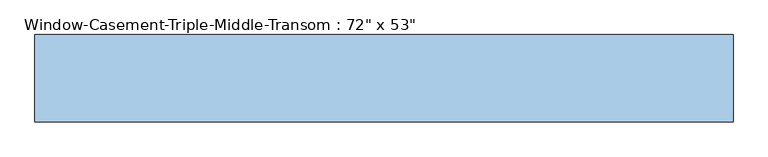
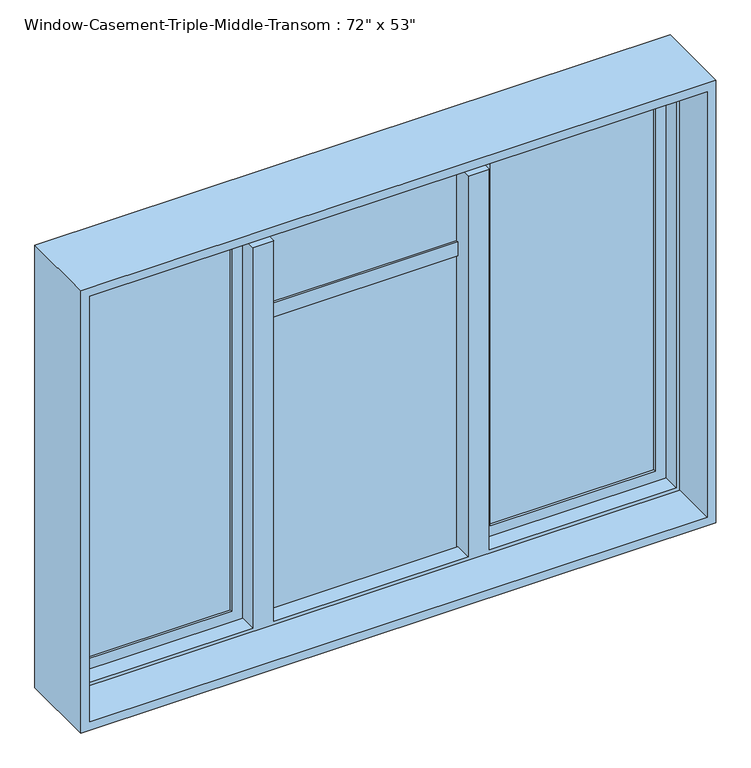
"""IFC4 building model written with IfcOpenShell, lengths in millimetres: window geometry."""

from ifc_helpers import new_model, si_unit, frame, origin, place, context, project, spatial, polyline, outline, extrude, faceted_brep, source, transform, mapped, element, save


def window_7a1f68bc(model_context):
    return source(origin(), model_context, "Body", "SolidModel", [
        extrude(outline(polyline([(2235.2, 330.2), (939.8, 330.2), (939.8, 889.0), (2235.2, 889.0), (2235.2, 330.2)]), holes=[polyline([(2193.3296875, 847.1296875), (981.6703125, 847.1296875), (981.6703125, 372.0703125), (2193.3296875, 372.0703125), (2193.3296875, 847.1296875)])]), frame((0.0, 73.025, 0.0), z_axis=(0.0, 1.0, 0.0), x_axis=(0.0, 0.0, 1.0)), (0.0, 0.0, 1.0), 31.75),
        extrude(outline(polyline([(2235.2, -889.0), (939.8, -889.0), (939.8, -330.2), (2235.2, -330.2), (2235.2, -889.0)]), holes=[polyline([(2193.3296875, -372.0703125), (981.6703125, -372.0703125), (981.6703125, -847.1296875), (2193.3296875, -847.1296875), (2193.3296875, -372.0703125)])]), frame((0.0, 73.025, 0.0), z_axis=(0.0, 1.0, 0.0), x_axis=(0.0, 0.0, 1.0)), (0.0, 0.0, 1.0), 31.75),
        extrude(outline(polyline([(-372.0703125, 98.425), (-372.0703125, 92.075), (-847.1296875, 92.075), (-847.1296875, 98.425), (-372.0703125, 98.425)])), frame((0.0, 0.0, 949.9203125), z_axis=(0.0, 0.0, 1.0), x_axis=(1.0, 0.0, 0.0)), (0.0, 0.0, 1.0), 1275.159375),
        extrude(outline(polyline([(-372.0703125, 85.725), (-372.0703125, 79.375), (-847.1296875, 79.375), (-847.1296875, 85.725), (-372.0703125, 85.725)])), frame((0.0, 0.0, 949.9203125), z_axis=(0.0, 0.0, 1.0), x_axis=(1.0, 0.0, 0.0)), (0.0, 0.0, 1.0), 1275.159375),
        extrude(outline(polyline([(847.1296875, 98.425), (847.1296875, 92.075), (372.0703125, 92.075), (372.0703125, 98.425), (847.1296875, 98.425)])), frame((0.0, 0.0, 949.9203125), z_axis=(0.0, 0.0, 1.0), x_axis=(1.0, 0.0, 0.0)), (0.0, 0.0, 1.0), 1275.159375),
        extrude(outline(polyline([(847.1296875, 85.725), (847.1296875, 79.375), (372.0703125, 79.375), (372.0703125, 85.725), (847.1296875, 85.725)])), frame((0.0, 0.0, 949.9203125), z_axis=(0.0, 0.0, 1.0), x_axis=(1.0, 0.0, 0.0)), (0.0, 0.0, 1.0), 1275.159375),
        extrude(outline(polyline([(279.4, 104.775), (279.4, 73.025), (-279.4, 73.025), (-279.4, 104.775), (279.4, 104.775)])), frame((0.0, 0.0, 1835.8048438), z_axis=(0.0, 0.0, 1.0), x_axis=(1.0, 0.0, 0.0)), (0.0, 0.0, 1.0), 41.8703125),
        extrude(outline(polyline([(279.4, 98.425), (279.4, 92.075), (-279.4, 92.075), (-279.4, 98.425), (279.4, 98.425)])), frame((0.0, 0.0, 939.8), z_axis=(0.0, 0.0, 1.0), x_axis=(1.0, 0.0, 0.0)), (0.0, 0.0, 1.0), 896.0048437),
        extrude(outline(polyline([(279.4, 85.725), (279.4, 79.375), (-279.4, 79.375), (-279.4, 85.725), (279.4, 85.725)])), frame((0.0, 0.0, 939.8), z_axis=(0.0, 0.0, 1.0), x_axis=(1.0, 0.0, 0.0)), (0.0, 0.0, 1.0), 896.0048437),
        extrude(outline(polyline([(279.4, 98.425), (279.4, 92.075), (-279.4, 92.075), (-279.4, 98.425), (279.4, 98.425)])), frame((0.0, 0.0, 1877.6751563), z_axis=(0.0, 0.0, 1.0), x_axis=(1.0, 0.0, 0.0)), (0.0, 0.0, 1.0), 357.5248438),
        extrude(outline(polyline([(279.4, 85.725), (279.4, 79.375), (-279.4, 79.375), (-279.4, 85.725), (279.4, 85.725)])), frame((0.0, 0.0, 1877.6751563), z_axis=(0.0, 0.0, 1.0), x_axis=(1.0, 0.0, 0.0)), (0.0, 0.0, 1.0), 357.5248438),
        faceted_brep([(-889.0, 73.025, 2235.2), (-889.0, 114.3, 2235.2), (889.0, 114.3, 2235.2), (889.0, 73.025, 2235.2), (-878.8796875, 22.225, 2225.0796875), (-878.8796875, 73.025, 2225.0796875), (878.8796875, 73.025, 2225.0796875), (878.8796875, 22.225, 2225.0796875), (-889.0, -114.3, 2235.2), (-889.0, 22.225, 2235.2), (889.0, 22.225, 2235.2), (889.0, -114.3, 2235.2), (-914.4, 114.3, 2260.6), (-914.4, -114.3, 2260.6), (914.4, -114.3, 2260.6), (914.4, 114.3, 2260.6), (889.0, 114.3, 939.8), (889.0, 73.025, 939.8), (878.8796875, 73.025, 949.9203125), (878.8796875, 22.225, 949.9203125), (889.0, 22.225, 939.8), (889.0, -114.3, 939.8), (914.4, -114.3, 914.4), (914.4, 114.3, 914.4), (330.2, 73.025, 939.8), (-889.0, 114.3, 939.8), (-889.0, 73.025, 939.8), (-330.2, 73.025, 939.8), (-330.2, 111.125, 939.8), (-279.4, 111.125, 939.8), (-279.4, 73.025, 939.8), (279.4, 73.025, 939.8), (279.4, 111.125, 939.8), (330.2, 111.125, 939.8), (340.3203125, 73.025, 949.9203125), (340.3203125, 22.225, 949.9203125), (-878.8796875, 73.025, 949.9203125), (-878.8796875, 22.225, 949.9203125), (-340.3203125, 22.225, 949.9203125), (-340.3203125, 73.025, 949.9203125), (279.4, 73.025, 949.9203125), (-279.4, 73.025, 949.9203125), (-279.4, 22.225, 949.9203125), (279.4, 22.225, 949.9203125), (-889.0, 22.225, 939.8), (-889.0, -114.3, 939.8), (-914.4, -114.3, 914.4), (-914.4, 114.3, 914.4), (330.2, 73.025, 2108.2), (340.3203125, 73.025, 2108.2), (-340.3203125, 73.025, 2108.2), (-330.2, 73.025, 2108.2), (-279.4, 111.125, 2108.2), (-330.2, 111.125, 2108.2), (-340.3203125, 22.225, 2108.2), (-279.4, 22.225, 2108.2), (330.2, 111.125, 2108.2), (279.4, 111.125, 2108.2), (279.4, 22.225, 2108.2), (340.3203125, 22.225, 2108.2)], [[[0, 1, 2, 3]], [[4, 5, 6, 7]], [[8, 9, 10, 11]], [[12, 13, 14, 15]], [[3, 2, 16, 17]], [[7, 6, 18, 19]], [[11, 10, 20, 21]], [[15, 14, 22, 23]], [[24, 17, 16, 25, 26, 27, 28, 29, 30, 31, 32, 33]], [[19, 18, 34, 35]], [[36, 37, 38, 39]], [[40, 41, 42, 43]], [[21, 20, 44, 45]], [[23, 22, 46, 47]], [[1, 0, 26, 25]], [[0, 3, 17, 24, 48, 49, 34, 18, 6, 5, 36, 39, 50, 51, 27, 26]], [[41, 40, 31, 30]], [[5, 4, 37, 36]], [[9, 8, 45, 44]], [[14, 13, 46, 22], [8, 11, 21, 45]], [[13, 12, 47, 46]], [[12, 15, 23, 47], [2, 1, 25, 16]], [[52, 53, 51, 50, 54, 55]], [[56, 57, 58, 59, 49, 48]], [[53, 52, 29, 28]], [[27, 51, 53, 28]], [[52, 55, 42, 41, 30, 29]], [[57, 56, 33, 32]], [[58, 57, 32, 31, 40, 43]], [[56, 48, 24, 33]], [[54, 50, 39, 38]], [[49, 59, 35, 34]], [[10, 9, 44, 20], [4, 7, 19, 35, 59, 58, 43, 42, 55, 54, 38, 37]]]),
    ])


if __name__ == "__main__":
    model = new_model("IFC4")
    model_context = context("Model", 3, world=origin())
    ifc_project = project(units=[si_unit("LENGTHUNIT", "METRE", prefix="MILLI")], contexts=[model_context])
    site = spatial("IfcSite", under=ifc_project)
    building = spatial("IfcBuilding", under=site)
    placement = place(None, origin())
    window_shape = window_7a1f68bc(model_context)
    element("IfcWindow", 1, ObjectType="Window-Casement-Triple-Middle-Transom : 72\" x 53\"", at=placement, inside=building, context=model_context, shape_type="MappedRepresentation", body=[
        mapped(window_shape, transform((0.0, 0.0, 0.0), x_axis=(1.0, 0.0, 0.0), y_axis=(0.0, 1.0, 0.0), z_axis=(0.0, 0.0, 1.0))),
    ])
    save(model, "model.ifc")

# Revit data of these elements
# Type "Window-Casement-Triple-Middle-Transom : 72\" x 53\""
#   Type Mark = "18"
#   Fire Rating = "0.5h"
#   Assembly Code = "B2020100"
#   Analytic Construction = "Double glazing - domestic"
#   Window Width = 2' - 0"
#   Window Inset [instance default] = 0' - 0 5/8"
#   Wall Thickness [instance default] = 0' - 6"
#   Visual Light Transmittance = 0.81
#   Transom Height Ratio = 0.3
#   Thermal Resistance (R) = 1.8146 (h·ft²·°F)/BTU
#   Solar Heat Gain Coefficient = 0.76
#   Rough Width = 6' - 0 1/2"
#   Rough Height = 4' - 5 1/2"
#   Heat Transfer Coefficient (U) = 0.5511 BTU/(h·ft²·°F)
#   Height = 4' - 5"
#   Transom Height = 1' - 3.9"
#   Frame Gap 3 [instance default] = 0' - 1 83/128"
#   Frame Gap 2 [instance default] = 0' - 0 5/8"
#   Frame Gap 1 = 0' - 1 51/128"
#   Default Sill Height = 3' - 0"
#   Width = 6' - 0"
#   Frame Material = Metal - Aluminum
#   Glass Panel Material = Glass
#   Wall Closure = (empty or 0)
# Element 1 (IfcWindow, "Window-Casement-Triple-Middle-Transom : 72\" x 53\"")
#   Wall Thickness = 0' - 9"
#   Materials on its faces: "Metal - Aluminum", "Glass"
# Materials
#   "Metal - Aluminum": class "Metal", colour RGB 247 247 247, transparency 0
#   "Glass": class "Glass", colour RGB 0 128 192, transparency 0.75, Description = "Soda Lime Glass", Cost = 0
